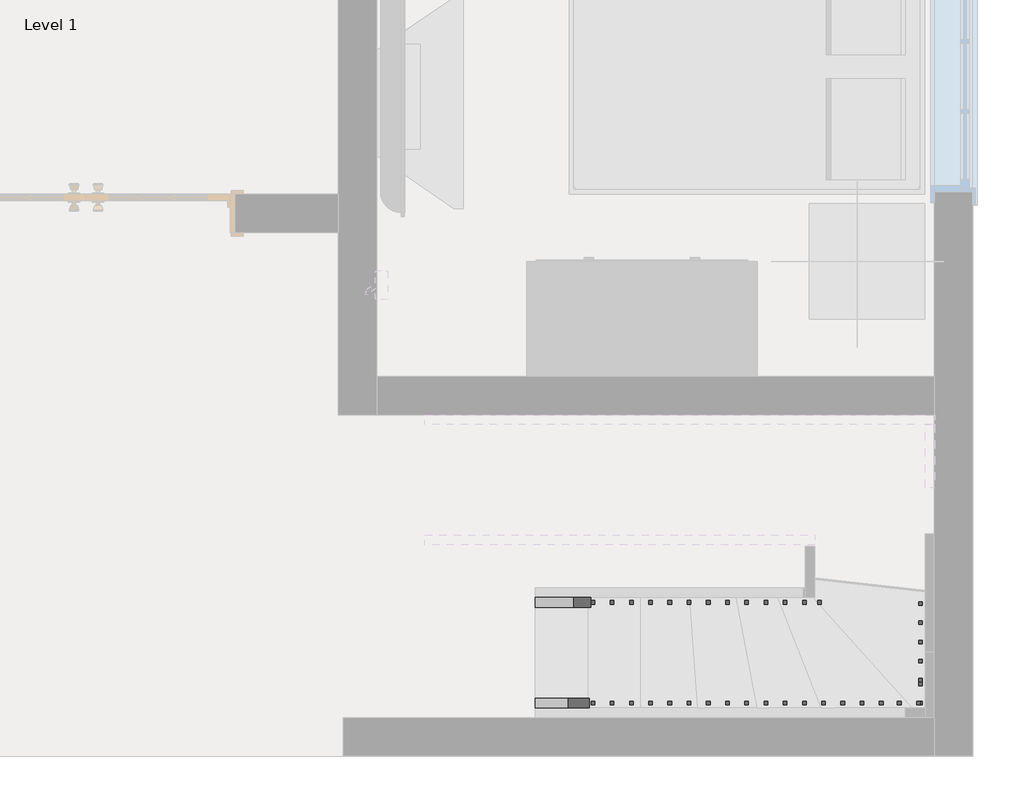
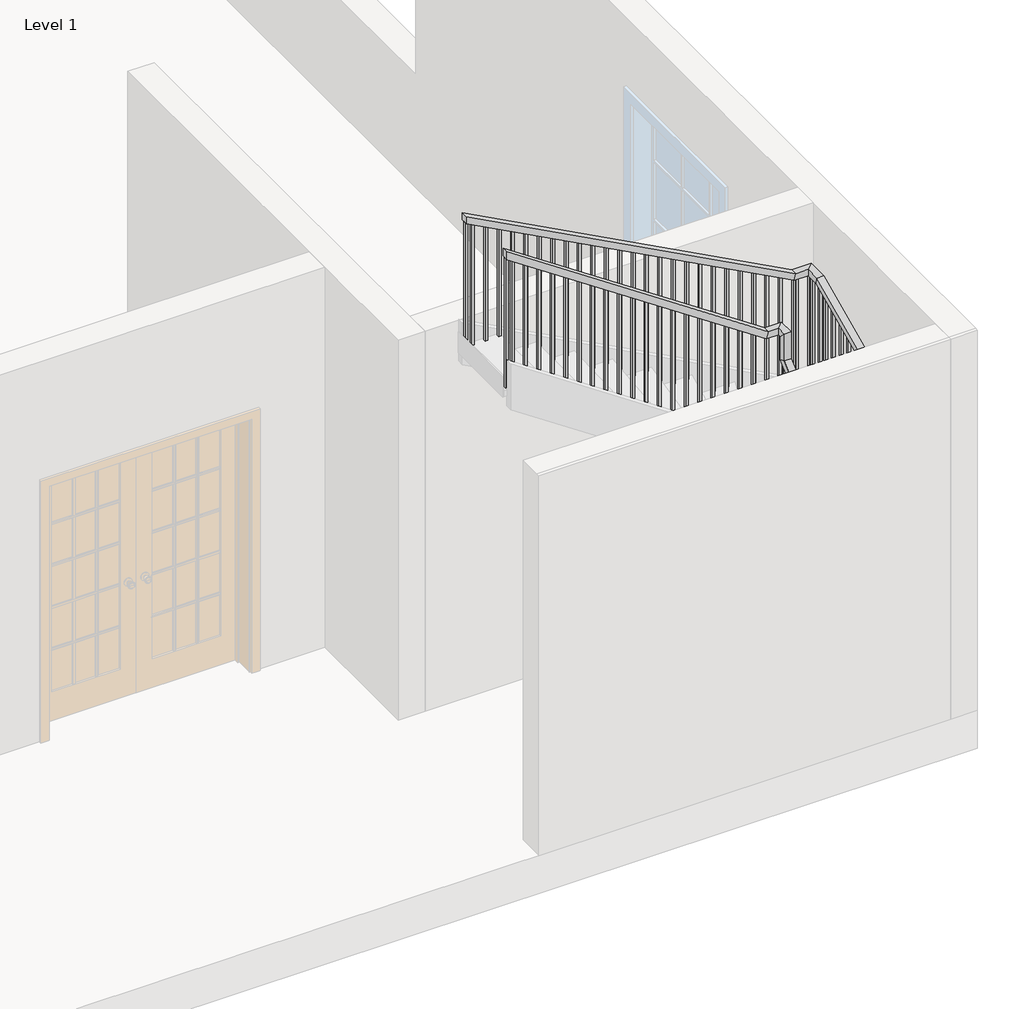
# One storey, part 2 of 3: 2 railings.
"""IFC4 building model written with IfcOpenShell, lengths in millimetres."""

from ifc_helpers import new_model, si_unit, frame, origin, place, context, project, spatial, polyline, outline, extrude, faceted_brep, element, save

model = new_model("IFC4")

# Units and contexts
model_context = context("Model", 3, world=origin())
ifc_project = project(units=[si_unit("LENGTHUNIT", "METRE", prefix="MILLI")], contexts=[model_context])

# Site, building, storey
site = spatial("IfcSite", under=ifc_project)
building = spatial("IfcBuilding", under=site)
storey = spatial("IfcBuildingStorey", under=building, Name="Level 1", Elevation=0.0)

# Railings
placement = place(None, origin())
element("IfcRailing", 1, ObjectType="Handrail - Rectangular", at=placement, inside=storey, context=model_context, shape_type="SolidModel", body=[
    faceted_brep([(376.3877765, 503.6595092, 1114.93083), (376.3877765, 503.6595092, 1058.2613171), (376.3877765, 452.8595092, 1058.2613171), (376.3877765, 452.8595092, 1114.93083), (2300.7380768, 503.6595092, 2066.3329014), (2312.6100281, 503.6595092, 2015.5329014), (2312.6100281, 452.8595092, 2015.5329014), (2300.7380768, 452.8595092, 2066.3329014), (2387.4275323, 503.6595092, 2015.5329014), (2387.4275323, 503.6595092, 2066.3329014), (2387.4275323, 599.1974434, 2066.3329014), (2387.4275323, 610.2822747, 2015.5329014), (2438.2275323, 452.8595092, 2015.5329014), (2438.2275323, 610.2822747, 2015.5329014), (2438.2275323, 452.8595092, 2066.3329014), (2438.2275323, 599.1974434, 2066.3329014), (2387.4275323, 1900.6595092, 2559.2104008), (2387.4275323, 1900.6595092, 2610.0104008), (2292.1444414, 1900.6595092, 2610.0104008), (2279.4506561, 1900.6595092, 2559.2104008), (2438.2275323, 1951.4595092, 2559.2104008), (2279.4506561, 1951.4595092, 2559.2104008), (2438.2275323, 1951.4595092, 2610.0104008), (2292.1444414, 1951.4595092, 2610.0104008), (2387.4275323, 1785.6740658, 2610.0104008), (2387.4275323, 1796.7588971, 2559.2104008), (2438.2275323, 1796.7588971, 2559.2104008), (2438.2275323, 1785.6740658, 2610.0104008), (-206.7168353, 1900.6595092, 3941.9973663), (-206.7168353, 1951.4595092, 3941.9973663), (-206.7168353, 1951.4595092, 3884.4311017), (-206.7168353, 1900.6595092, 3884.4311017)], [[[0, 1, 2, 3]], [[1, 0, 4, 5]], [[2, 1, 5, 6]], [[3, 2, 6, 7]], [[0, 3, 7, 4]], [[8, 9, 10, 11]], [[12, 8, 11, 13]], [[14, 12, 13, 15]], [[9, 14, 15, 10]], [[16, 17, 18, 19]], [[20, 16, 19, 21]], [[22, 20, 21, 23]], [[17, 22, 23, 18]], [[5, 4, 9, 8]], [[6, 5, 8, 12]], [[7, 6, 12, 14]], [[4, 7, 14, 9]], [[11, 10, 24, 25]], [[13, 11, 25, 26]], [[15, 13, 26, 27]], [[10, 15, 27, 24]], [[25, 24, 17, 16]], [[26, 25, 16, 20]], [[27, 26, 20, 22]], [[24, 27, 22, 17]], [[28, 29, 30, 31]], [[19, 18, 28, 31]], [[21, 19, 31, 30]], [[23, 21, 30, 29]], [[18, 23, 29, 28]]]),
    extrude(outline(polyline([(3847.1257862, -136.7305586), (3857.280152, -155.7805586), (2878.6666667, -155.7805586), (2878.6666667, -136.7305586), (3847.1257862, -136.7305586)])), frame((0.0, 1916.5345092, 0.0), z_axis=(0.0, 1.0, 0.0), x_axis=(0.0, 0.0, 1.0)), (0.0, 0.0, 1.0), 19.05),
    extrude(outline(polyline([(3792.9691681, -35.1305586), (3803.123534, -54.1805586), (2878.6666667, -54.1805586), (2878.6666667, -35.1305586), (3792.9691681, -35.1305586)])), frame((0.0, 1916.5345092, 0.0), z_axis=(0.0, 1.0, 0.0), x_axis=(0.0, 0.0, 1.0)), (0.0, 0.0, 1.0), 19.05),
    extrude(outline(polyline([(3738.8125501, 66.4694414), (3748.966916, 47.4194414), (2878.6666667, 47.4194414), (2878.6666667, 66.4694414), (3738.8125501, 66.4694414)])), frame((0.0, 1916.5345092, 0.0), z_axis=(0.0, 1.0, 0.0), x_axis=(0.0, 0.0, 1.0)), (0.0, 0.0, 1.0), 19.05),
    extrude(outline(polyline([(3684.655932, 168.0694414), (3694.8102979, 149.0194414), (2709.3333333, 149.0194414), (2709.3333333, 168.0694414), (3684.655932, 168.0694414)])), frame((0.0, 1916.5345092, 0.0), z_axis=(0.0, 1.0, 0.0), x_axis=(0.0, 0.0, 1.0)), (0.0, 0.0, 1.0), 19.05),
    extrude(outline(polyline([(3630.499314, 269.6694414), (3640.6536799, 250.6194414), (2709.3333333, 250.6194414), (2709.3333333, 269.6694414), (3630.499314, 269.6694414)])), frame((0.0, 1916.5345092, 0.0), z_axis=(0.0, 1.0, 0.0), x_axis=(0.0, 0.0, 1.0)), (0.0, 0.0, 1.0), 19.05),
    extrude(outline(polyline([(3576.342696, 371.2694414), (3586.4970619, 352.2194414), (2540.0, 352.2194414), (2540.0, 371.2694414), (3576.342696, 371.2694414)])), frame((0.0, 1916.5345092, 0.0), z_axis=(0.0, 1.0, 0.0), x_axis=(0.0, 0.0, 1.0)), (0.0, 0.0, 1.0), 19.05),
    extrude(outline(polyline([(3522.1860779, 472.8694414), (3532.3404438, 453.8194414), (2540.0, 453.8194414), (2540.0, 472.8694414), (3522.1860779, 472.8694414)])), frame((0.0, 1916.5345092, 0.0), z_axis=(0.0, 1.0, 0.0), x_axis=(0.0, 0.0, 1.0)), (0.0, 0.0, 1.0), 19.05),
    extrude(outline(polyline([(3468.0294599, 574.4694414), (3478.1838258, 555.4194414), (2540.0, 555.4194414), (2540.0, 574.4694414), (3468.0294599, 574.4694414)])), frame((0.0, 1916.5345092, 0.0), z_axis=(0.0, 1.0, 0.0), x_axis=(0.0, 0.0, 1.0)), (0.0, 0.0, 1.0), 19.05),
    extrude(outline(polyline([(3413.8728419, 676.0694414), (3424.0272077, 657.0194414), (2370.6666667, 657.0194414), (2370.6666667, 676.0694414), (3413.8728419, 676.0694414)])), frame((0.0, 1916.5345092, 0.0), z_axis=(0.0, 1.0, 0.0), x_axis=(0.0, 0.0, 1.0)), (0.0, 0.0, 1.0), 19.05),
    extrude(outline(polyline([(3359.7162238, 777.6694414), (3369.8705897, 758.6194414), (2370.6666667, 758.6194414), (2370.6666667, 777.6694414), (3359.7162238, 777.6694414)])), frame((0.0, 1916.5345092, 0.0), z_axis=(0.0, 1.0, 0.0), x_axis=(0.0, 0.0, 1.0)), (0.0, 0.0, 1.0), 19.05),
    extrude(outline(polyline([(3305.5596058, 879.2694414), (3315.7139717, 860.2194414), (2370.6666667, 860.2194414), (2370.6666667, 879.2694414), (3305.5596058, 879.2694414)])), frame((0.0, 1916.5345092, 0.0), z_axis=(0.0, 1.0, 0.0), x_axis=(0.0, 0.0, 1.0)), (0.0, 0.0, 1.0), 19.05),
    extrude(outline(polyline([(3251.4029877, 980.8694414), (3261.5573536, 961.8194414), (2201.3333333, 961.8194414), (2201.3333333, 980.8694414), (3251.4029877, 980.8694414)])), frame((0.0, 1916.5345092, 0.0), z_axis=(0.0, 1.0, 0.0), x_axis=(0.0, 0.0, 1.0)), (0.0, 0.0, 1.0), 19.05),
    extrude(outline(polyline([(3197.2463697, 1082.4694414), (3207.4007356, 1063.4194414), (2201.3333333, 1063.4194414), (2201.3333333, 1082.4694414), (3197.2463697, 1082.4694414)])), frame((0.0, 1916.5345092, 0.0), z_axis=(0.0, 1.0, 0.0), x_axis=(0.0, 0.0, 1.0)), (0.0, 0.0, 1.0), 19.05),
    extrude(outline(polyline([(3143.0897517, 1184.0694414), (3153.2441175, 1165.0194414), (2201.3333333, 1165.0194414), (2201.3333333, 1184.0694414), (3143.0897517, 1184.0694414)])), frame((0.0, 1916.5345092, 0.0), z_axis=(0.0, 1.0, 0.0), x_axis=(0.0, 0.0, 1.0)), (0.0, 0.0, 1.0), 19.05),
    extrude(outline(polyline([(3088.9331336, 1285.6694414), (3099.0874995, 1266.6194414), (2032.0, 1266.6194414), (2032.0, 1285.6694414), (3088.9331336, 1285.6694414)])), frame((0.0, 1916.5345092, 0.0), z_axis=(0.0, 1.0, 0.0), x_axis=(0.0, 0.0, 1.0)), (0.0, 0.0, 1.0), 19.05),
    extrude(outline(polyline([(3034.7765156, 1387.2694414), (3044.9308815, 1368.2194414), (2032.0, 1368.2194414), (2032.0, 1387.2694414), (3034.7765156, 1387.2694414)])), frame((0.0, 1916.5345092, 0.0), z_axis=(0.0, 1.0, 0.0), x_axis=(0.0, 0.0, 1.0)), (0.0, 0.0, 1.0), 19.05),
    extrude(outline(polyline([(2980.6198975, 1488.8694414), (2990.7742634, 1469.8194414), (2032.0, 1469.8194414), (2032.0, 1488.8694414), (2980.6198975, 1488.8694414)])), frame((0.0, 1916.5345092, 0.0), z_axis=(0.0, 1.0, 0.0), x_axis=(0.0, 0.0, 1.0)), (0.0, 0.0, 1.0), 19.05),
    extrude(outline(polyline([(2926.4632795, 1590.4694414), (2936.6176454, 1571.4194414), (1862.6666667, 1571.4194414), (1862.6666667, 1590.4694414), (2926.4632795, 1590.4694414)])), frame((0.0, 1916.5345092, 0.0), z_axis=(0.0, 1.0, 0.0), x_axis=(0.0, 0.0, 1.0)), (0.0, 0.0, 1.0), 19.05),
    extrude(outline(polyline([(2872.3066615, 1692.0694414), (2882.4610273, 1673.0194414), (1862.6666667, 1673.0194414), (1862.6666667, 1692.0694414), (2872.3066615, 1692.0694414)])), frame((0.0, 1916.5345092, 0.0), z_axis=(0.0, 1.0, 0.0), x_axis=(0.0, 0.0, 1.0)), (0.0, 0.0, 1.0), 19.05),
    extrude(outline(polyline([(2818.1500434, 1793.6694414), (2828.3044093, 1774.6194414), (1862.6666667, 1774.6194414), (1862.6666667, 1793.6694414), (2818.1500434, 1793.6694414)])), frame((0.0, 1916.5345092, 0.0), z_axis=(0.0, 1.0, 0.0), x_axis=(0.0, 0.0, 1.0)), (0.0, 0.0, 1.0), 19.05),
    extrude(outline(polyline([(2763.9934254, 1895.2694414), (2774.1477913, 1876.2194414), (1693.3333333, 1876.2194414), (1693.3333333, 1895.2694414), (2763.9934254, 1895.2694414)])), frame((0.0, 1916.5345092, 0.0), z_axis=(0.0, 1.0, 0.0), x_axis=(0.0, 0.0, 1.0)), (0.0, 0.0, 1.0), 19.05),
    extrude(outline(polyline([(2709.8368074, 1996.8694414), (2719.9911732, 1977.8194414), (1693.3333333, 1977.8194414), (1693.3333333, 1996.8694414), (2709.8368074, 1996.8694414)])), frame((0.0, 1916.5345092, 0.0), z_axis=(0.0, 1.0, 0.0), x_axis=(0.0, 0.0, 1.0)), (0.0, 0.0, 1.0), 19.05),
    extrude(outline(polyline([(2655.6801893, 2098.4694414), (2665.8345552, 2079.4194414), (1693.3333333, 2079.4194414), (1693.3333333, 2098.4694414), (2655.6801893, 2098.4694414)])), frame((0.0, 1916.5345092, 0.0), z_axis=(0.0, 1.0, 0.0), x_axis=(0.0, 0.0, 1.0)), (0.0, 0.0, 1.0), 19.05),
    extrude(outline(polyline([(2601.5235713, 2200.0694414), (2611.6779372, 2181.0194414), (1693.3333333, 2181.0194414), (1693.3333333, 2200.0694414), (2601.5235713, 2200.0694414)])), frame((0.0, 1916.5345092, 0.0), z_axis=(0.0, 1.0, 0.0), x_axis=(0.0, 0.0, 1.0)), (0.0, 0.0, 1.0), 19.05),
    extrude(outline(polyline([(2320.7525323, 1935.5845092), (2320.7525323, 1916.5345092), (2301.7025323, 1916.5345092), (2301.7025323, 1935.5845092), (2320.7525323, 1935.5845092)])), frame((0.0, 0.0, 1524.0), z_axis=(0.0, 0.0, 1.0), x_axis=(1.0, 0.0, 0.0)), (0.0, 0.0, 1.0), 1035.2104008),
    extrude(outline(polyline([(2422.3525323, 1877.7490658), (2403.3025323, 1877.7490658), (2403.3025323, 1896.7990658), (2422.3525323, 1896.7990658), (2422.3525323, 1877.7490658)])), frame((0.0, 0.0, 1524.0), z_axis=(0.0, 0.0, 1.0), x_axis=(1.0, 0.0, 0.0)), (0.0, 0.0, 1.0), 1035.2104008),
    extrude(outline(polyline([(1707.2724434, 2518.2051501), (1726.3224434, 2526.9344045), (1726.3224434, 1524.0), (1707.2724434, 1524.0), (1707.2724434, 2518.2051501)])), frame((2403.3025323, 0.0, 0.0), z_axis=(1.0, 0.0, 0.0), x_axis=(0.0, 1.0, 0.0)), (0.0, 0.0, 1.0), 19.05),
    extrude(outline(polyline([(1605.6724434, 2471.6491262), (1624.7224434, 2480.3783807), (1624.7224434, 1524.0), (1605.6724434, 1524.0), (1605.6724434, 2471.6491262)])), frame((2403.3025323, 0.0, 0.0), z_axis=(1.0, 0.0, 0.0), x_axis=(0.0, 1.0, 0.0)), (0.0, 0.0, 1.0), 19.05),
    extrude(outline(polyline([(1504.0724434, 2425.0931023), (1523.1224434, 2433.8223568), (1523.1224434, 1524.0), (1504.0724434, 1524.0), (1504.0724434, 2425.0931023)])), frame((2403.3025323, 0.0, 0.0), z_axis=(1.0, 0.0, 0.0), x_axis=(0.0, 1.0, 0.0)), (0.0, 0.0, 1.0), 19.05),
    extrude(outline(polyline([(1402.4724434, 2378.5370785), (1421.5224434, 2387.2663329), (1421.5224434, 1524.0), (1402.4724434, 1524.0), (1402.4724434, 2378.5370785)])), frame((2403.3025323, 0.0, 0.0), z_axis=(1.0, 0.0, 0.0), x_axis=(0.0, 1.0, 0.0)), (0.0, 0.0, 1.0), 19.05),
    extrude(outline(polyline([(1300.8724434, 2331.9810546), (1319.9224434, 2340.7103091), (1319.9224434, 1354.6666667), (1300.8724434, 1354.6666667), (1300.8724434, 2331.9810546)])), frame((2403.3025323, 0.0, 0.0), z_axis=(1.0, 0.0, 0.0), x_axis=(0.0, 1.0, 0.0)), (0.0, 0.0, 1.0), 19.05),
    extrude(outline(polyline([(1199.2724434, 2285.4250307), (1218.3224434, 2294.1542852), (1218.3224434, 1354.6666667), (1199.2724434, 1354.6666667), (1199.2724434, 2285.4250307)])), frame((2403.3025323, 0.0, 0.0), z_axis=(1.0, 0.0, 0.0), x_axis=(0.0, 1.0, 0.0)), (0.0, 0.0, 1.0), 19.05),
    extrude(outline(polyline([(1097.6724434, 2238.8690069), (1116.7224434, 2247.5982614), (1116.7224434, 1354.6666667), (1097.6724434, 1354.6666667), (1097.6724434, 2238.8690069)])), frame((2403.3025323, 0.0, 0.0), z_axis=(1.0, 0.0, 0.0), x_axis=(0.0, 1.0, 0.0)), (0.0, 0.0, 1.0), 19.05),
    extrude(outline(polyline([(996.0724434, 2192.312983), (1015.1224434, 2201.0422375), (1015.1224434, 1185.3333333), (996.0724434, 1185.3333333), (996.0724434, 2192.312983)])), frame((2403.3025323, 0.0, 0.0), z_axis=(1.0, 0.0, 0.0), x_axis=(0.0, 1.0, 0.0)), (0.0, 0.0, 1.0), 19.05),
    extrude(outline(polyline([(894.4724434, 2145.7569592), (913.5224434, 2154.4862136), (913.5224434, 1185.3333333), (894.4724434, 1185.3333333), (894.4724434, 2145.7569592)])), frame((2403.3025323, 0.0, 0.0), z_axis=(1.0, 0.0, 0.0), x_axis=(0.0, 1.0, 0.0)), (0.0, 0.0, 1.0), 19.05),
    extrude(outline(polyline([(792.8724434, 2099.2009353), (811.9224434, 2107.9301898), (811.9224434, 1185.3333333), (792.8724434, 1185.3333333), (792.8724434, 2099.2009353)])), frame((2403.3025323, 0.0, 0.0), z_axis=(1.0, 0.0, 0.0), x_axis=(0.0, 1.0, 0.0)), (0.0, 0.0, 1.0), 19.05),
    extrude(outline(polyline([(691.2724434, 2052.6449114), (710.3224434, 2061.3741659), (710.3224434, 1185.3333333), (691.2724434, 1185.3333333), (691.2724434, 2052.6449114)])), frame((2403.3025323, 0.0, 0.0), z_axis=(1.0, 0.0, 0.0), x_axis=(0.0, 1.0, 0.0)), (0.0, 0.0, 1.0), 19.05),
    extrude(outline(polyline([(2422.3525323, 570.3345092), (2403.3025323, 570.3345092), (2403.3025323, 589.3845092), (2422.3525323, 589.3845092), (2422.3525323, 570.3345092)])), frame((0.0, 0.0, 1185.3333333), z_axis=(0.0, 0.0, 1.0), x_axis=(1.0, 0.0, 0.0)), (0.0, 0.0, 1.0), 830.199568),
    extrude(outline(polyline([(2392.8130768, 468.7345092), (2392.8130768, 487.7845092), (2411.8630768, 487.7845092), (2411.8630768, 468.7345092), (2392.8130768, 468.7345092)])), frame((0.0, 0.0, 1185.3333333), z_axis=(0.0, 0.0, 1.0), x_axis=(1.0, 0.0, 0.0)), (0.0, 0.0, 1.0), 830.199568),
    extrude(outline(polyline([(1967.1323332, 2214.7127765), (1957.7139807, 2195.6627765), (1016.0, 2195.6627765), (1016.0, 2214.7127765), (1967.1323332, 2214.7127765)])), frame((0.0, 468.7345092, 0.0), z_axis=(0.0, 1.0, 0.0), x_axis=(0.0, 0.0, 1.0)), (0.0, 0.0, 1.0), 19.05),
    extrude(outline(polyline([(1916.9011198, 2113.1127765), (1907.4827673, 2094.0627765), (1016.0, 2094.0627765), (1016.0, 2113.1127765), (1916.9011198, 2113.1127765)])), frame((0.0, 468.7345092, 0.0), z_axis=(0.0, 1.0, 0.0), x_axis=(0.0, 0.0, 1.0)), (0.0, 0.0, 1.0), 19.05),
    extrude(outline(polyline([(1866.6699065, 2011.5127765), (1857.251554, 1992.4627765), (1016.0, 1992.4627765), (1016.0, 2011.5127765), (1866.6699065, 2011.5127765)])), frame((0.0, 468.7345092, 0.0), z_axis=(0.0, 1.0, 0.0), x_axis=(0.0, 0.0, 1.0)), (0.0, 0.0, 1.0), 19.05),
    extrude(outline(polyline([(1816.4386932, 1909.9127765), (1807.0203407, 1890.8627765), (1016.0, 1890.8627765), (1016.0, 1909.9127765), (1816.4386932, 1909.9127765)])), frame((0.0, 468.7345092, 0.0), z_axis=(0.0, 1.0, 0.0), x_axis=(0.0, 0.0, 1.0)), (0.0, 0.0, 1.0), 19.05),
    extrude(outline(polyline([(1766.2074799, 1808.3127765), (1756.7891274, 1789.2627765), (846.6666667, 1789.2627765), (846.6666667, 1808.3127765), (1766.2074799, 1808.3127765)])), frame((0.0, 468.7345092, 0.0), z_axis=(0.0, 1.0, 0.0), x_axis=(0.0, 0.0, 1.0)), (0.0, 0.0, 1.0), 19.05),
    extrude(outline(polyline([(1715.9762665, 1706.7127765), (1706.557914, 1687.6627765), (846.6666667, 1687.6627765), (846.6666667, 1706.7127765), (1715.9762665, 1706.7127765)])), frame((0.0, 468.7345092, 0.0), z_axis=(0.0, 1.0, 0.0), x_axis=(0.0, 0.0, 1.0)), (0.0, 0.0, 1.0), 19.05),
    extrude(outline(polyline([(1665.7450532, 1605.1127765), (1656.3267007, 1586.0627765), (846.6666667, 1586.0627765), (846.6666667, 1605.1127765), (1665.7450532, 1605.1127765)])), frame((0.0, 468.7345092, 0.0), z_axis=(0.0, 1.0, 0.0), x_axis=(0.0, 0.0, 1.0)), (0.0, 0.0, 1.0), 19.05),
    extrude(outline(polyline([(1615.5138399, 1503.5127765), (1606.0954874, 1484.4627765), (677.3333333, 1484.4627765), (677.3333333, 1503.5127765), (1615.5138399, 1503.5127765)])), frame((0.0, 468.7345092, 0.0), z_axis=(0.0, 1.0, 0.0), x_axis=(0.0, 0.0, 1.0)), (0.0, 0.0, 1.0), 19.05),
    extrude(outline(polyline([(1565.2826266, 1401.9127765), (1555.8642741, 1382.8627765), (677.3333333, 1382.8627765), (677.3333333, 1401.9127765), (1565.2826266, 1401.9127765)])), frame((0.0, 468.7345092, 0.0), z_axis=(0.0, 1.0, 0.0), x_axis=(0.0, 0.0, 1.0)), (0.0, 0.0, 1.0), 19.05),
    extrude(outline(polyline([(1515.0514132, 1300.3127765), (1505.6330607, 1281.2627765), (677.3333333, 1281.2627765), (677.3333333, 1300.3127765), (1515.0514132, 1300.3127765)])), frame((0.0, 468.7345092, 0.0), z_axis=(0.0, 1.0, 0.0), x_axis=(0.0, 0.0, 1.0)), (0.0, 0.0, 1.0), 19.05),
    extrude(outline(polyline([(1464.8201999, 1198.7127765), (1455.4018474, 1179.6627765), (508.0, 1179.6627765), (508.0, 1198.7127765), (1464.8201999, 1198.7127765)])), frame((0.0, 468.7345092, 0.0), z_axis=(0.0, 1.0, 0.0), x_axis=(0.0, 0.0, 1.0)), (0.0, 0.0, 1.0), 19.05),
    extrude(outline(polyline([(1414.5889866, 1097.1127765), (1405.1706341, 1078.0627765), (508.0, 1078.0627765), (508.0, 1097.1127765), (1414.5889866, 1097.1127765)])), frame((0.0, 468.7345092, 0.0), z_axis=(0.0, 1.0, 0.0), x_axis=(0.0, 0.0, 1.0)), (0.0, 0.0, 1.0), 19.05),
    extrude(outline(polyline([(1364.3577733, 995.5127765), (1354.9394208, 976.4627765), (508.0, 976.4627765), (508.0, 995.5127765), (1364.3577733, 995.5127765)])), frame((0.0, 468.7345092, 0.0), z_axis=(0.0, 1.0, 0.0), x_axis=(0.0, 0.0, 1.0)), (0.0, 0.0, 1.0), 19.05),
    extrude(outline(polyline([(1314.1265599, 893.9127765), (1304.7082074, 874.8627765), (338.6666667, 874.8627765), (338.6666667, 893.9127765), (1314.1265599, 893.9127765)])), frame((0.0, 468.7345092, 0.0), z_axis=(0.0, 1.0, 0.0), x_axis=(0.0, 0.0, 1.0)), (0.0, 0.0, 1.0), 19.05),
    extrude(outline(polyline([(1263.8953466, 792.3127765), (1254.4769941, 773.2627765), (338.6666667, 773.2627765), (338.6666667, 792.3127765), (1263.8953466, 792.3127765)])), frame((0.0, 468.7345092, 0.0), z_axis=(0.0, 1.0, 0.0), x_axis=(0.0, 0.0, 1.0)), (0.0, 0.0, 1.0), 19.05),
    extrude(outline(polyline([(1213.6641333, 690.7127765), (1204.2457808, 671.6627765), (338.6666667, 671.6627765), (338.6666667, 690.7127765), (1213.6641333, 690.7127765)])), frame((0.0, 468.7345092, 0.0), z_axis=(0.0, 1.0, 0.0), x_axis=(0.0, 0.0, 1.0)), (0.0, 0.0, 1.0), 19.05),
    extrude(outline(polyline([(1163.43292, 589.1127765), (1154.0145675, 570.0627765), (169.3333333, 570.0627765), (169.3333333, 589.1127765), (1163.43292, 589.1127765)])), frame((0.0, 468.7345092, 0.0), z_axis=(0.0, 1.0, 0.0), x_axis=(0.0, 0.0, 1.0)), (0.0, 0.0, 1.0), 19.05),
    extrude(outline(polyline([(1113.2017066, 487.5127765), (1103.7833541, 468.4627765), (169.3333333, 468.4627765), (169.3333333, 487.5127765), (1113.2017066, 487.5127765)])), frame((0.0, 468.7345092, 0.0), z_axis=(0.0, 1.0, 0.0), x_axis=(0.0, 0.0, 1.0)), (0.0, 0.0, 1.0), 19.05),
    extrude(outline(polyline([(2301.6694414, 1935.5845092), (2301.6694414, 1916.5345092), (2282.6194414, 1916.5345092), (2282.6194414, 1935.5845092), (2301.6694414, 1935.5845092)])), frame((0.0, 0.0, 1524.0), z_axis=(0.0, 0.0, 1.0), x_axis=(1.0, 0.0, 0.0)), (0.0, 0.0, 1.0), 1035.2104008),
    extrude(outline(polyline([(2422.3525323, 1916.5345092), (2403.3025323, 1916.5345092), (2403.3025323, 1935.5845092), (2422.3525323, 1935.5845092), (2422.3525323, 1916.5345092)])), frame((0.0, 0.0, 1524.0), z_axis=(0.0, 0.0, 1.0), x_axis=(1.0, 0.0, 0.0)), (0.0, 0.0, 1.0), 1035.2104008),
    extrude(outline(polyline([(1776.1490658, 2549.766387), (1795.1990658, 2558.4956415), (1795.1990658, 1524.0), (1776.1490658, 1524.0), (1776.1490658, 2549.766387)])), frame((2403.3025323, 0.0, 0.0), z_axis=(1.0, 0.0, 0.0), x_axis=(0.0, 1.0, 0.0)), (0.0, 0.0, 1.0), 19.05),
    extrude(outline(polyline([(2422.3525323, 589.6724434), (2403.3025323, 589.6724434), (2403.3025323, 608.7224434), (2422.3525323, 608.7224434), (2422.3525323, 589.6724434)])), frame((0.0, 0.0, 1185.3333333), z_axis=(0.0, 0.0, 1.0), x_axis=(1.0, 0.0, 0.0)), (0.0, 0.0, 1.0), 830.199568),
    extrude(outline(polyline([(2403.3025323, 468.7345092), (2403.3025323, 487.7845092), (2422.3525323, 487.7845092), (2422.3525323, 468.7345092), (2403.3025323, 468.7345092)])), frame((0.0, 0.0, 1185.3333333), z_axis=(0.0, 0.0, 1.0), x_axis=(1.0, 0.0, 0.0)), (0.0, 0.0, 1.0), 830.199568),
    extrude(outline(polyline([(2014.3725646, 2310.2630768), (2004.9542122, 2291.2130768), (1016.0, 2291.2130768), (1016.0, 2310.2630768), (2014.3725646, 2310.2630768)])), frame((0.0, 468.7345092, 0.0), z_axis=(0.0, 1.0, 0.0), x_axis=(0.0, 0.0, 1.0)), (0.0, 0.0, 1.0), 19.05),
    extrude(outline(polyline([(3874.2767358, -187.6668353), (3884.4311017, -206.7168353), (2878.6666667, -206.7168353), (2878.6666667, -187.6668353), (3874.2767358, -187.6668353)])), frame((0.0, 1916.5345092, 0.0), z_axis=(0.0, 1.0, 0.0), x_axis=(0.0, 0.0, 1.0)), (0.0, 0.0, 1.0), 19.05),
    extrude(outline(polyline([(1067.6796696, 395.4377765), (1058.2613171, 376.3877765), (169.3333333, 376.3877765), (169.3333333, 395.4377765), (1067.6796696, 395.4377765)])), frame((0.0, 468.7345092, 0.0), z_axis=(0.0, 1.0, 0.0), x_axis=(0.0, 0.0, 1.0)), (0.0, 0.0, 1.0), 19.05),
])
element("IfcRailing", 2, ObjectType="Handrail - Rectangular", at=placement, inside=storey, context=model_context, shape_type="SolidModel", body=[
    faceted_brep([(376.3877765, 1037.0595092, 1054.1431537), (376.3877765, 1037.0595092, 991.7832482), (376.3877765, 986.2595092, 991.7832482), (376.3877765, 986.2595092, 1054.1431537), (1777.8275323, 1037.0595092, 2051.9216769), (1828.6275323, 1037.0595092, 2025.7296828), (1828.6275323, 986.2595092, 2025.7296828), (1777.8275323, 986.2595092, 2051.9216769), (1854.0275323, 1132.6679233, 2222.5348555), (1854.0275323, 1113.2595092, 2273.3348555), (1854.0275323, 1291.0595092, 2432.4139433), (1854.0275323, 1341.8595092, 2409.7002473), (1904.8275323, 1132.6679233, 2222.5348555), (1904.8275323, 1341.8595092, 2409.7002473), (1904.8275323, 1113.2595092, 2273.3348555), (1904.8275323, 1291.0595092, 2432.4139433), (-206.7168353, 1367.2595092, 3980.9638314), (-206.7168353, 1418.0595092, 3980.9638314), (-206.7168353, 1418.0595092, 3919.7448897), (-206.7168353, 1367.2595092, 3919.7448897), (1762.3347369, 1367.2595092, 2595.5530227), (1777.8275323, 1367.2595092, 2646.3530227), (1762.3347369, 1418.0595092, 2595.5530227), (1777.8275323, 1418.0595092, 2646.3530227), (1777.8275323, 1037.0595092, 2273.3348555), (1828.6275323, 1037.0595092, 2222.5348555), (1828.6275323, 986.2595092, 2222.5348555), (1777.8275323, 986.2595092, 2273.3348555), (1854.0275323, 1037.0595092, 2273.3348555), (1854.0275323, 1037.0595092, 2222.5348555), (1904.8275323, 986.2595092, 2222.5348555), (1904.8275323, 986.2595092, 2273.3348555), (1854.0275323, 1291.0595092, 2646.3530227), (1854.0275323, 1341.8595092, 2595.5530227), (1904.8275323, 1341.8595092, 2595.5530227), (1904.8275323, 1291.0595092, 2646.3530227), (1854.0275323, 1367.2595092, 2646.3530227), (1854.0275323, 1367.2595092, 2595.5530227), (1904.8275323, 1418.0595092, 2595.5530227), (1904.8275323, 1418.0595092, 2646.3530227)], [[[0, 1, 2, 3]], [[1, 0, 4, 5]], [[2, 1, 5, 6]], [[3, 2, 6, 7]], [[0, 3, 7, 4]], [[8, 9, 10, 11]], [[12, 8, 11, 13]], [[14, 12, 13, 15]], [[9, 14, 15, 10]], [[16, 17, 18, 19]], [[20, 21, 16, 19]], [[22, 20, 19, 18]], [[23, 22, 18, 17]], [[21, 23, 17, 16]], [[5, 4, 24, 25]], [[6, 5, 25, 26]], [[7, 6, 26, 27]], [[4, 7, 27, 24]], [[25, 24, 28, 29]], [[26, 25, 29, 30]], [[27, 26, 30, 31]], [[24, 27, 31, 28]], [[29, 28, 9, 8]], [[30, 29, 8, 12]], [[31, 30, 12, 14]], [[28, 31, 14, 9]], [[11, 10, 32, 33]], [[13, 11, 33, 34]], [[15, 13, 34, 35]], [[10, 15, 35, 32]], [[33, 32, 36, 37]], [[34, 33, 37, 38]], [[35, 34, 38, 39]], [[32, 35, 39, 36]], [[37, 36, 21, 20]], [[38, 37, 20, 22]], [[39, 38, 22, 23]], [[36, 39, 23, 21]]]),
    extrude(outline(polyline([(3889.7382588, -162.0974677), (2878.6666667, -162.0974677), (2878.6666667, -143.0474677), (3876.9270885, -143.0474677), (3889.7382588, -162.0974677)])), frame((0.0, 1383.1345092, 0.0), z_axis=(0.0, 1.0, 0.0), x_axis=(0.0, 0.0, 1.0)), (0.0, 0.0, 1.0), 19.05),
    extrude(outline(polyline([(3821.4120171, -60.4974677), (2878.6666667, -60.4974677), (2878.6666667, -41.4474677), (3808.6008467, -41.4474677), (3821.4120171, -60.4974677)])), frame((0.0, 1383.1345092, 0.0), z_axis=(0.0, 1.0, 0.0), x_axis=(0.0, 0.0, 1.0)), (0.0, 0.0, 1.0), 19.05),
    extrude(outline(polyline([(3753.0857753, 41.1025323), (2878.6666667, 41.1025323), (2878.6666667, 60.1525323), (3740.274605, 60.1525323), (3753.0857753, 41.1025323)])), frame((0.0, 1383.1345092, 0.0), z_axis=(0.0, 1.0, 0.0), x_axis=(0.0, 0.0, 1.0)), (0.0, 0.0, 1.0), 19.05),
    extrude(outline(polyline([(3684.7595336, 142.7025323), (2709.3333333, 142.7025323), (2709.3333333, 161.7525323), (3671.9483633, 161.7525323), (3684.7595336, 142.7025323)])), frame((0.0, 1383.1345092, 0.0), z_axis=(0.0, 1.0, 0.0), x_axis=(0.0, 0.0, 1.0)), (0.0, 0.0, 1.0), 19.05),
    extrude(outline(polyline([(3616.4332919, 244.3025323), (2709.3333333, 244.3025323), (2709.3333333, 263.3525323), (3603.6221216, 263.3525323), (3616.4332919, 244.3025323)])), frame((0.0, 1383.1345092, 0.0), z_axis=(0.0, 1.0, 0.0), x_axis=(0.0, 0.0, 1.0)), (0.0, 0.0, 1.0), 19.05),
    extrude(outline(polyline([(3548.1070502, 345.9025323), (2540.0, 345.9025323), (2540.0, 364.9525323), (3535.2958799, 364.9525323), (3548.1070502, 345.9025323)])), frame((0.0, 1383.1345092, 0.0), z_axis=(0.0, 1.0, 0.0), x_axis=(0.0, 0.0, 1.0)), (0.0, 0.0, 1.0), 19.05),
    extrude(outline(polyline([(3479.7808085, 447.5025323), (2540.0, 447.5025323), (2540.0, 466.5525323), (3466.9696382, 466.5525323), (3479.7808085, 447.5025323)])), frame((0.0, 1383.1345092, 0.0), z_axis=(0.0, 1.0, 0.0), x_axis=(0.0, 0.0, 1.0)), (0.0, 0.0, 1.0), 19.05),
    extrude(outline(polyline([(3411.4545668, 549.1025323), (2540.0, 549.1025323), (2540.0, 568.1525323), (3398.6433964, 568.1525323), (3411.4545668, 549.1025323)])), frame((0.0, 1383.1345092, 0.0), z_axis=(0.0, 1.0, 0.0), x_axis=(0.0, 0.0, 1.0)), (0.0, 0.0, 1.0), 19.05),
    extrude(outline(polyline([(3343.1283251, 650.7025323), (2370.6666667, 650.7025323), (2370.6666667, 669.7525323), (3330.3171547, 669.7525323), (3343.1283251, 650.7025323)])), frame((0.0, 1383.1345092, 0.0), z_axis=(0.0, 1.0, 0.0), x_axis=(0.0, 0.0, 1.0)), (0.0, 0.0, 1.0), 19.05),
    extrude(outline(polyline([(3274.8020833, 752.3025323), (2370.6666667, 752.3025323), (2370.6666667, 771.3525323), (3261.990913, 771.3525323), (3274.8020833, 752.3025323)])), frame((0.0, 1383.1345092, 0.0), z_axis=(0.0, 1.0, 0.0), x_axis=(0.0, 0.0, 1.0)), (0.0, 0.0, 1.0), 19.05),
    extrude(outline(polyline([(3206.4758416, 853.9025323), (2370.6666667, 853.9025323), (2370.6666667, 872.9525323), (3193.6646713, 872.9525323), (3206.4758416, 853.9025323)])), frame((0.0, 1383.1345092, 0.0), z_axis=(0.0, 1.0, 0.0), x_axis=(0.0, 0.0, 1.0)), (0.0, 0.0, 1.0), 19.05),
    extrude(outline(polyline([(3138.1495999, 955.5025323), (2201.3333333, 955.5025323), (2201.3333333, 974.5525323), (3125.3384296, 974.5525323), (3138.1495999, 955.5025323)])), frame((0.0, 1383.1345092, 0.0), z_axis=(0.0, 1.0, 0.0), x_axis=(0.0, 0.0, 1.0)), (0.0, 0.0, 1.0), 19.05),
    extrude(outline(polyline([(3069.8233582, 1057.1025323), (2201.3333333, 1057.1025323), (2201.3333333, 1076.1525323), (3057.0121879, 1076.1525323), (3069.8233582, 1057.1025323)])), frame((0.0, 1383.1345092, 0.0), z_axis=(0.0, 1.0, 0.0), x_axis=(0.0, 0.0, 1.0)), (0.0, 0.0, 1.0), 19.05),
    extrude(outline(polyline([(3001.4971165, 1158.7025323), (2032.0, 1158.7025323), (2032.0, 1177.7525323), (2988.6859461, 1177.7525323), (3001.4971165, 1158.7025323)])), frame((0.0, 1383.1345092, 0.0), z_axis=(0.0, 1.0, 0.0), x_axis=(0.0, 0.0, 1.0)), (0.0, 0.0, 1.0), 19.05),
    extrude(outline(polyline([(2933.1708748, 1260.3025323), (2032.0, 1260.3025323), (2032.0, 1279.3525323), (2920.3597044, 1279.3525323), (2933.1708748, 1260.3025323)])), frame((0.0, 1383.1345092, 0.0), z_axis=(0.0, 1.0, 0.0), x_axis=(0.0, 0.0, 1.0)), (0.0, 0.0, 1.0), 19.05),
    extrude(outline(polyline([(2864.844633, 1361.9025323), (2032.0, 1361.9025323), (2032.0, 1380.9525323), (2852.0334627, 1380.9525323), (2864.844633, 1361.9025323)])), frame((0.0, 1383.1345092, 0.0), z_axis=(0.0, 1.0, 0.0), x_axis=(0.0, 0.0, 1.0)), (0.0, 0.0, 1.0), 19.05),
    extrude(outline(polyline([(2796.5183913, 1463.5025323), (1862.6666667, 1463.5025323), (1862.6666667, 1482.5525323), (2783.707221, 1482.5525323), (2796.5183913, 1463.5025323)])), frame((0.0, 1383.1345092, 0.0), z_axis=(0.0, 1.0, 0.0), x_axis=(0.0, 0.0, 1.0)), (0.0, 0.0, 1.0), 19.05),
    extrude(outline(polyline([(2728.1921496, 1565.1025323), (1862.6666667, 1565.1025323), (1862.6666667, 1584.1525323), (2715.3809793, 1584.1525323), (2728.1921496, 1565.1025323)])), frame((0.0, 1383.1345092, 0.0), z_axis=(0.0, 1.0, 0.0), x_axis=(0.0, 0.0, 1.0)), (0.0, 0.0, 1.0), 19.05),
    extrude(outline(polyline([(2659.8659079, 1666.7025323), (1693.3333333, 1666.7025323), (1693.3333333, 1685.7525323), (2647.0547376, 1685.7525323), (2659.8659079, 1666.7025323)])), frame((0.0, 1383.1345092, 0.0), z_axis=(0.0, 1.0, 0.0), x_axis=(0.0, 0.0, 1.0)), (0.0, 0.0, 1.0), 19.05),
    extrude(outline(polyline([(1787.3525323, 1383.1345092), (1768.3025323, 1383.1345092), (1768.3025323, 1402.1845092), (1787.3525323, 1402.1845092), (1787.3525323, 1383.1345092)])), frame((0.0, 0.0, 1693.3333333), z_axis=(0.0, 0.0, 1.0), x_axis=(1.0, 0.0, 0.0)), (0.0, 0.0, 1.0), 902.2196894),
    extrude(outline(polyline([(1325.9845092, 2395.4967574), (1325.9845092, 1524.0), (1306.9345092, 1524.0), (1306.9345092, 2378.4525694), (1325.9845092, 2395.4967574)])), frame((1869.9025323, 0.0, 0.0), z_axis=(1.0, 0.0, 0.0), x_axis=(0.0, 1.0, 0.0)), (0.0, 0.0, 1.0), 19.05),
    extrude(outline(polyline([(1224.3845092, 2304.5944215), (1224.3845092, 1354.6666667), (1205.3345092, 1354.6666667), (1205.3345092, 2287.5502335), (1224.3845092, 2304.5944215)])), frame((1869.9025323, 0.0, 0.0), z_axis=(1.0, 0.0, 0.0), x_axis=(0.0, 1.0, 0.0)), (0.0, 0.0, 1.0), 19.05),
    extrude(outline(polyline([(1869.9025323, 1103.7345092), (1869.9025323, 1122.7845092), (1888.9525323, 1122.7845092), (1888.9525323, 1103.7345092), (1869.9025323, 1103.7345092)])), frame((0.0, 0.0, 1354.6666667), z_axis=(0.0, 0.0, 1.0), x_axis=(1.0, 0.0, 0.0)), (0.0, 0.0, 1.0), 867.8681888),
    extrude(outline(polyline([(1997.7032852, 1789.2627765), (1016.0, 1789.2627765), (1016.0, 1808.3127765), (2011.266252, 1808.3127765), (1997.7032852, 1789.2627765)])), frame((0.0, 1002.1345092, 0.0), z_axis=(0.0, 1.0, 0.0), x_axis=(0.0, 0.0, 1.0)), (0.0, 0.0, 1.0), 19.05),
    extrude(outline(polyline([(1925.3674623, 1687.6627765), (1016.0, 1687.6627765), (1016.0, 1706.7127765), (1938.9304291, 1706.7127765), (1925.3674623, 1687.6627765)])), frame((0.0, 1002.1345092, 0.0), z_axis=(0.0, 1.0, 0.0), x_axis=(0.0, 0.0, 1.0)), (0.0, 0.0, 1.0), 19.05),
    extrude(outline(polyline([(1853.0316394, 1586.0627765), (846.6666667, 1586.0627765), (846.6666667, 1605.1127765), (1866.5946062, 1605.1127765), (1853.0316394, 1586.0627765)])), frame((0.0, 1002.1345092, 0.0), z_axis=(0.0, 1.0, 0.0), x_axis=(0.0, 0.0, 1.0)), (0.0, 0.0, 1.0), 19.05),
    extrude(outline(polyline([(1780.6958165, 1484.4627765), (846.6666667, 1484.4627765), (846.6666667, 1503.5127765), (1794.2587833, 1503.5127765), (1780.6958165, 1484.4627765)])), frame((0.0, 1002.1345092, 0.0), z_axis=(0.0, 1.0, 0.0), x_axis=(0.0, 0.0, 1.0)), (0.0, 0.0, 1.0), 19.05),
    extrude(outline(polyline([(1708.3599936, 1382.8627765), (677.3333333, 1382.8627765), (677.3333333, 1401.9127765), (1721.9229604, 1401.9127765), (1708.3599936, 1382.8627765)])), frame((0.0, 1002.1345092, 0.0), z_axis=(0.0, 1.0, 0.0), x_axis=(0.0, 0.0, 1.0)), (0.0, 0.0, 1.0), 19.05),
    extrude(outline(polyline([(1636.0241708, 1281.2627765), (677.3333333, 1281.2627765), (677.3333333, 1300.3127765), (1649.5871376, 1300.3127765), (1636.0241708, 1281.2627765)])), frame((0.0, 1002.1345092, 0.0), z_axis=(0.0, 1.0, 0.0), x_axis=(0.0, 0.0, 1.0)), (0.0, 0.0, 1.0), 19.05),
    extrude(outline(polyline([(1563.6883479, 1179.6627765), (508.0, 1179.6627765), (508.0, 1198.7127765), (1577.2513147, 1198.7127765), (1563.6883479, 1179.6627765)])), frame((0.0, 1002.1345092, 0.0), z_axis=(0.0, 1.0, 0.0), x_axis=(0.0, 0.0, 1.0)), (0.0, 0.0, 1.0), 19.05),
    extrude(outline(polyline([(1491.352525, 1078.0627765), (508.0, 1078.0627765), (508.0, 1097.1127765), (1504.9154918, 1097.1127765), (1491.352525, 1078.0627765)])), frame((0.0, 1002.1345092, 0.0), z_axis=(0.0, 1.0, 0.0), x_axis=(0.0, 0.0, 1.0)), (0.0, 0.0, 1.0), 19.05),
    extrude(outline(polyline([(1419.0167021, 976.4627765), (508.0, 976.4627765), (508.0, 995.5127765), (1432.5796689, 995.5127765), (1419.0167021, 976.4627765)])), frame((0.0, 1002.1345092, 0.0), z_axis=(0.0, 1.0, 0.0), x_axis=(0.0, 0.0, 1.0)), (0.0, 0.0, 1.0), 19.05),
    extrude(outline(polyline([(1346.6808792, 874.8627765), (338.6666667, 874.8627765), (338.6666667, 893.9127765), (1360.243846, 893.9127765), (1346.6808792, 874.8627765)])), frame((0.0, 1002.1345092, 0.0), z_axis=(0.0, 1.0, 0.0), x_axis=(0.0, 0.0, 1.0)), (0.0, 0.0, 1.0), 19.05),
    extrude(outline(polyline([(1274.3450563, 773.2627765), (338.6666667, 773.2627765), (338.6666667, 792.3127765), (1287.9080231, 792.3127765), (1274.3450563, 773.2627765)])), frame((0.0, 1002.1345092, 0.0), z_axis=(0.0, 1.0, 0.0), x_axis=(0.0, 0.0, 1.0)), (0.0, 0.0, 1.0), 19.05),
    extrude(outline(polyline([(1202.0092335, 671.6627765), (338.6666667, 671.6627765), (338.6666667, 690.7127765), (1215.5722003, 690.7127765), (1202.0092335, 671.6627765)])), frame((0.0, 1002.1345092, 0.0), z_axis=(0.0, 1.0, 0.0), x_axis=(0.0, 0.0, 1.0)), (0.0, 0.0, 1.0), 19.05),
    extrude(outline(polyline([(1129.6734106, 570.0627765), (169.3333333, 570.0627765), (169.3333333, 589.1127765), (1143.2363774, 589.1127765), (1129.6734106, 570.0627765)])), frame((0.0, 1002.1345092, 0.0), z_axis=(0.0, 1.0, 0.0), x_axis=(0.0, 0.0, 1.0)), (0.0, 0.0, 1.0), 19.05),
    extrude(outline(polyline([(1057.3375877, 468.4627765), (169.3333333, 468.4627765), (169.3333333, 487.5127765), (1070.9005545, 487.5127765), (1057.3375877, 468.4627765)])), frame((0.0, 1002.1345092, 0.0), z_axis=(0.0, 1.0, 0.0), x_axis=(0.0, 0.0, 1.0)), (0.0, 0.0, 1.0), 19.05),
    extrude(outline(polyline([(1888.9525323, 1383.1345092), (1869.9025323, 1383.1345092), (1869.9025323, 1402.1845092), (1888.9525323, 1402.1845092), (1888.9525323, 1383.1345092)])), frame((0.0, 0.0, 1524.0), z_axis=(0.0, 0.0, 1.0), x_axis=(1.0, 0.0, 0.0)), (0.0, 0.0, 1.0), 1071.5530227),
    extrude(outline(polyline([(1869.9025323, 1002.1345092), (1869.9025323, 1021.1845092), (1888.9525323, 1021.1845092), (1888.9525323, 1002.1345092), (1869.9025323, 1002.1345092)])), frame((0.0, 0.0, 1185.3333333), z_axis=(0.0, 0.0, 1.0), x_axis=(1.0, 0.0, 0.0)), (0.0, 0.0, 1.0), 1037.2015222),
    extrude(outline(polyline([(3919.7448897, -206.7168353), (2878.6666667, -206.7168353), (2878.6666667, -187.6668353), (3906.9337193, -187.6668353), (3919.7448897, -206.7168353)])), frame((0.0, 1383.1345092, 0.0), z_axis=(0.0, 1.0, 0.0), x_axis=(0.0, 0.0, 1.0)), (0.0, 0.0, 1.0), 19.05),
    extrude(outline(polyline([(991.7832482, 376.3877765), (169.3333333, 376.3877765), (169.3333333, 395.4377765), (1005.346215, 395.4377765), (991.7832482, 376.3877765)])), frame((0.0, 1002.1345092, 0.0), z_axis=(0.0, 1.0, 0.0), x_axis=(0.0, 0.0, 1.0)), (0.0, 0.0, 1.0), 19.05),
])

save(model, "model.ifc")

# Revit data of these elements
# Type "Handrail - Rectangular"
#   Assembly Code = "C2010400"
#   built-in parameter 1008612 = 0.0416667 (stored number, unit not read)
#   built-in parameter 1008611 = 0.0416667 (stored number, unit not read)
#   built-in parameter 1008609 = 0.333333 (stored number, unit not read)
#   built-in parameter 1008604 = 0.166667 (stored number, unit not read)
#   built-in parameter 1008603 = 0.166667 (stored number, unit not read)
#   Railing Height = 3' - 0"
#   built-in parameter 1008630 = 2
#   built-in parameter 1008610 = 2
#   built-in parameter 1008618 = Baluster - Square : 3/4"
# Elements 1, 2 (IfcRailing, "Handrail - Rectangular")
#   Phase Created = New Construction
